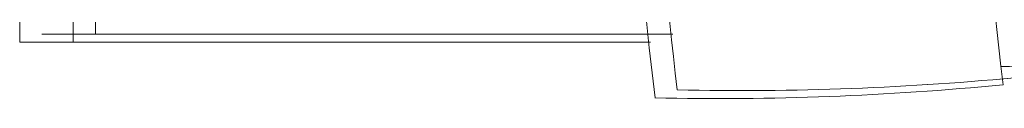
# Model space of a CAD drawing. Units: inches. Extents: x 1962 to 2771, y 1245 to 2660.
# Tile 24 of 114: x 2094 to 2116, y 1850 to 1852. Entities that reach past the tile are written whole.
import ezdxf

# ---------------------------------------------------------------- set-up
doc = ezdxf.new("R2010")
doc.units = ezdxf.units.IN
doc.layers.add('A-FURN', color=8, linetype='Continuous', lineweight=13)

# ---------------------------------------------------------------- blocks, each defined once
blk = doc.blocks.new('BED-PLAN')
for p, q in [((1.727, 2.945), (1.727, 40.933)), ((1.727, 2.945), (1.727, 40.933)), ((0, 2.764), (0, 40.751)), ((1.219, 2.764), (1.219, 40.752)), ((1.219, 2.763), (1.219, 40.751)), ((14.904, 2.945), (0.508, 2.945)), ((14.904, 2.945), (0.508, 2.945)), ((14.396, 2.764), (0, 2.764)), ((14.396, 2.763), (0, 2.763))]:
    blk.add_line(p, q)
for centre, radius, start, end in [((124.254, 14.115), 102.556, 171.78449, 186.90062), ((124.254, 14.115), 102.556, 171.78449, 186.90062), ((124.762, 14.297), 102.556, 171.78449, 186.90062), ((124.762, 14.296), 102.556, 171.78449, 186.90062), ((145.219, 17.161), 131.131, 176.08655, 186.78213), ((145.219, 17.161), 131.131, 176.08655, 186.78213), ((144.711, 16.979), 131.131, 176.08655, 186.78213), ((144.711, 16.979), 131.131, 176.08655, 186.78213), ((24.78, -132.989), 135.218, 88.4762, 91.00819), ((24.78, -132.989), 135.218, 88.4762, 91.00819), ((16.482, 67.877), 66.218, 268.72178, 275.60397), ((16.483, 67.877), 66.218, 268.72178, 275.60397), ((15.974, 67.695), 66.218, 268.72178, 275.60397), ((15.974, 67.695), 66.218, 268.72178, 275.60397)]:
    blk.add_arc(centre, radius, start, end)

msp = doc.modelspace()

# ---------------------------------------------------------------- block references
at = {"layer": 'A-FURN'}
msp.add_blockref('BED-PLAN', (2093.6551, 1848.7344), dxfattribs=at)

doc.saveas('drawing.dxf')
